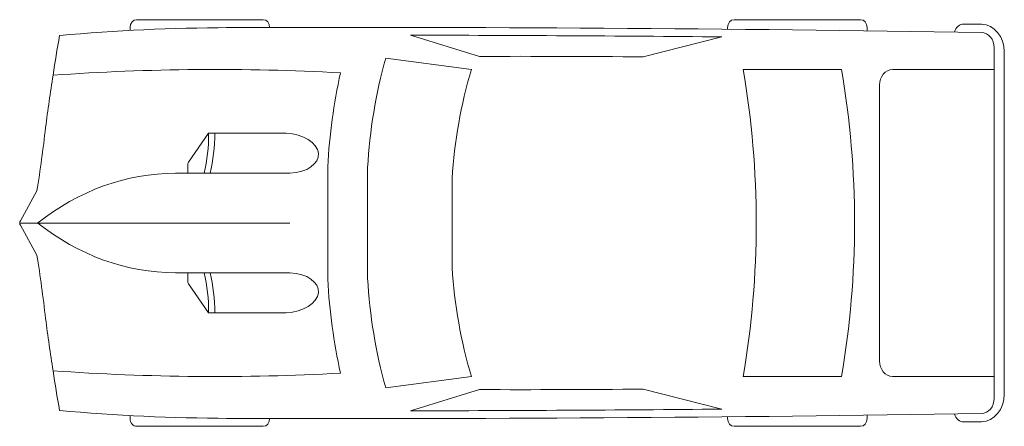
# Model space of a CAD drawing. Units: inches. Extents: x 1662 to 23131, y 1265 to 19127.
# Tile 8 of 26: x 15887 to 16075, y 8213 to 8291. Entities that reach past the tile are written whole.
import ezdxf

# ---------------------------------------------------------------- set-up
doc = ezdxf.new("R2010")
doc.units = ezdxf.units.IN
doc.layers.add('A-SITE-VEHC', color=8, linetype='Continuous', lineweight=18)

# ---------------------------------------------------------------- blocks, each defined once
blk = doc.blocks.new('*U66')
for p, q in [((1182.5, 987.8), (567.7, 987.8)), ((3472.1, 987.8), (4086.9, 987.8)), ((536, 950.2), (536, 935.5)), ((1214.1, 949.7), (1214.1, 950.2)), ((2234.8, 809.5), (1898.9, 912.4)), ((3440.5, 941.7), (3440.5, 950.2)), ((4118.5, 950.2), (4118.5, 934.1)), ((3411.6, 904.3), (3029.9, 807.2)), ((4736.4, -850.9), (4736.4, 850.9)), ((4785.3, -832.1), (4785.3, 832.1)), ((1778.8, 801), (2194.7, 745.5)), ((3515.9, 745.5), (3994.1, 745.5)), ((4736.4, 745.5), (4242, 745.5)), ((4178.7, 670.3), (4178.7, -670.3)), ((819.6, 295.3), (917.7, 436.1)), ((917.7, 436.1), (1293.8, 436.1)), ((756.2, 241.4), (1312.8, 241.4)), ((815.9, 241.4), (815.9, 283.3)), ((1496.5, -273.7), (1496.5, 273.7)), ((1690.4, -267.4), (1690.4, 267.4)), ((4736.4, -267.4), (4736.4, 267.4)), ((2101.5, 215.8), (2101.5, -215.8)), ((83, 155.7), (2.6, 10.3)), ((0, 0), (1312.8, 0)), ((2.6, -10.3), (83, -155.7)), ((756.2, -241.4), (1312.8, -241.4)), ((815.9, -241.4), (815.9, -283.3)), ((819.6, -295.3), (917.7, -436.1)), ((917.7, -436.1), (1293.8, -436.1)), ((2194.7, -745.5), (1778.8, -801)), ((3994.1, -745.5), (3515.9, -745.5)), ((4242, -745.5), (4736.4, -745.5)), ((2234.8, -809.5), (1898.9, -912.4)), ((3411.6, -904.3), (3029.9, -807.2)), ((536, -950.2), (536, -935.5)), ((1214.1, -949.7), (1214.1, -950.2)), ((3440.5, -941.7), (3440.5, -950.2)), ((4118.5, -950.2), (4118.5, -934.1)), ((1182.5, -987.8), (567.7, -987.8)), ((3472.1, -987.8), (4086.9, -987.8))]:
    blk.add_line(p, q)
for centre, major_axis, ratio, start_param, end_param in [((567.7, 950.2), (0, -37.6), 0.842304, 3.141593, 4.712389), ((1182.5, 950.2), (0, 37.6), 0.842304, -1.570796, 0), ((3472.1, 950.2), (0, -37.6), 0.842304, 3.141593, 4.712389), ((4086.9, 950.2), (0, 37.6), 0.842304, -1.570796, 0), ((4588, 910.3), (0, 56.4), 0.842304, -0.013017, 1.249894), ((1637.8, -268131.5), (0, 269121), 0.842304, -0.013397, -0.013017), ((4673.1, 832.1), (0, -133.3), 0.842304, 1.570796, 3.128196), ((6757.2, -699.1), (0, 7958), 0.842304, 1.367076, 1.39176), ((1046.3, -12467.9), (0, 13417.1), 0.842304, 0.00281, 0.075598), ((1637.8, -268112.7), (0, 269062.9), 0.842304, -0.013397, 0.002797), ((1637.8, -268112.7), (0, -269025.3), 0.842304, 3.133765, 3.140441), ((4673.1, 850.9), (0, -75.2), 0.842304, 1.570796, 3.128196), ((3436.4, 136.8), (0, 2077), 0.842304, 1.245306, 1.50788), ((2433, -93125.4), (0, -93935.2), 0.842304, 3.134049, 3.144098), ((6583, -699.1), (0, -7754.7), 0.842304, 4.528606, 4.561838), ((951.8, -15086.6), (0, -15832.5), 0.842304, 3.096046, 3.200911), ((3413.8, 136.8), (0, -2280.3), 0.842304, 4.449482, 4.652344), ((3799.7, 71.1), (0, -2021.3), 0.842304, 4.372215, 4.640744), ((433.9, 0), (0, 3734.3), 0.842304, 4.511394, 4.913384), ((912, 0), (0, 3734.3), 0.842304, 4.511394, 4.913384), ((4242, 670.3), (0, 75.2), 0.842304, 0, 1.570796), ((-5194.2, 1330.9), (0, -6374.4), 0.842304, 1.385369, 1.434372), ((331.1, 432), (0, 696.4), 0.842304, 4.435146, 4.718221), ((360.7, 432), (0, 696.4), 0.842304, 4.435146, 4.718221), ((1290.1, 338.8), (161, -9.1), 0.603834, -1.395552, 1.581315), ((831.8, 283.3), (0, 18.8), 0.842304, 0.879714, 1.570796), ((756.2, -1185.2), (0, 1426.7), 0.842304, 0, 0.590319), ((15.8, 0), (0, -18.8), 0.842304, 4.131459, 5.293319), ((756.2, 1185.2), (0, 1426.7), 0.842304, 2.551274, 3.141593), ((-5194.2, -1330.9), (0, 6374.4), 0.842304, -1.434372, -1.385369), ((3799.7, -71.1), (0, -2021.3), 0.842304, -1.499151, -1.230623), ((831.8, -283.3), (0, -18.8), 0.842304, 4.712389, 5.403472), ((331.1, -432), (0, -696.4), 0.842304, 1.564964, 1.848039), ((360.7, -432), (0, -696.4), 0.842304, 1.564964, 1.848039), ((3413.8, -136.8), (0, -2280.3), 0.842304, -1.510751, -1.307889), ((3436.4, -136.8), (0, -2077), 0.842304, -1.50788, -1.245306), ((6583, 699.1), (0, 7754.7), 0.842304, 1.721348, 1.754579), ((4242, -670.3), (0, -75.2), 0.842304, 4.712389, 6.283185), ((6757.2, 699.1), (0, 7958), 0.842304, 1.749832, 1.774517), ((951.8, 15086.6), (0, -15832.5), 0.842304, -0.059319, 0.045547), ((2433, 93125.4), (0, -93935.2), 0.842304, -0.002505, 0.007544), ((4673.1, -850.9), (0, 75.2), 0.842304, 3.15499, 4.712389), ((4673.1, -832.1), (0, -133.3), 0.842304, 0.013397, 1.570796), ((1637.8, 268112.7), (0, -269025.3), 0.842304, 0.001152, 0.007828), ((1046.3, 12467.9), (0, -13417.1), 0.842304, -0.075598, -0.00281), ((567.7, -950.2), (0, 37.6), 0.842304, 1.570796, 3.141593), ((1637.8, 268112.7), (0, 269062.9), 0.842304, 3.138796, 3.15499), ((1182.5, -950.2), (0, -37.6), 0.842304, 0, 1.570796), ((3472.1, -950.2), (0, -37.6), 0.842304, -1.570796, 0), ((4086.9, -950.2), (0, 37.6), 0.842304, 3.141593, 4.712389), ((4588, -910.3), (0, -56.4), 0.842304, -1.249894, 0.013017), ((1637.8, 268131.5), (0, 269121), 0.842304, 3.15461, 3.15499)]:
    blk.add_ellipse(centre, major_axis=major_axis, ratio=ratio, start_param=start_param, end_param=end_param)
at = {"extrusion": (0, 0, -1)}
blk.add_ellipse((1290.1, -338.8), major_axis=(161, 9.1), ratio=0.603834, start_param=-1.395552, end_param=1.581315, dxfattribs=at)

msp = doc.modelspace()

# ---------------------------------------------------------------- block references
at = {"layer": 'A-SITE-VEHC', "xscale": 0.0393700787401575, "yscale": 0.0393700787401575, "zscale": 0.0393700787401575}
msp.add_blockref('*U66', (15886.991, 8252.351), dxfattribs=at)

doc.saveas('drawing.dxf')
